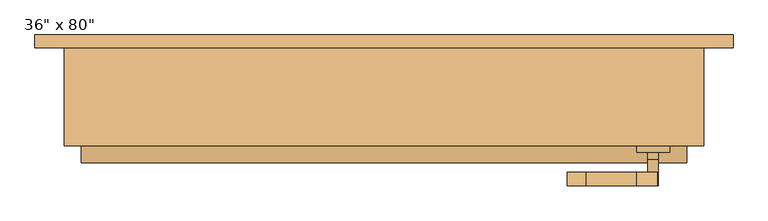
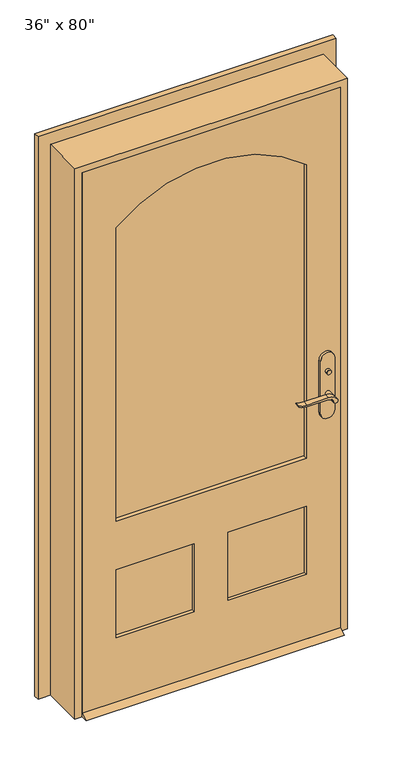
"""IFC4 building model written with IfcOpenShell, lengths in millimetres: door geometry."""

from ifc_helpers import new_model, si_unit, point, frame, frame_2d, origin, place, context, project, spatial, polyline, circle_curve, trimmed, segment, composite_curve, outline, extrude, faceted_brep, source, transform, mapped, element, save


def door_19287a7a(model_context):
    return source(origin(), model_context, "Body", "SolidModel", [
        extrude(outline(polyline([(-33.9718823, 12.7), (-8.5718823, 0.0), (-94.2968823, 0.0), (-68.8968823, 12.7), (-33.9718823, 12.7)])), frame((-457.2, 0.0, 0.0), z_axis=(1.0, 0.0, 0.0), x_axis=(0.0, 1.0, 0.0)), (0.0, 0.0, 1.0), 914.4),
        extrude(outline(polyline([(411.4, -13.9718823), (411.4, -23.9718823), (401.4, -23.9718823), (401.4, -13.9718823), (411.4, -13.9718823)])), frame((0.0, 0.0, 981.9), z_axis=(0.0, 0.0, 1.0), x_axis=(1.0, 0.0, 0.0)), (0.0, 0.0, 1.0), 30.0),
        extrude(outline(composite_curve([segment(trimmed(circle_curve(frame_2d((996.9, 406.4)), 8.0), [point((996.9, 398.4))], [point((996.9, 414.4))], False, "CARTESIAN"), True, "CONTINUOUS"), segment(trimmed(circle_curve(frame_2d((996.9, 406.4)), 8.0), [point((996.9, 414.4))], [point((996.9, 398.4))], False, "CARTESIAN"), True, "CONTINUOUS")], self_intersect=False)), frame((0.0, -88.8968823, 0.0), z_axis=(0.0, 1.0, 0.0), x_axis=(0.0, 0.0, 1.0)), (0.0, 0.0, 1.0), 10.0),
        extrude(outline(composite_curve([segment(trimmed(circle_curve(frame_2d((897.1555521, 382.7324871)), 37.2832219), [point((919.0523287, 412.9081363))], [point((934.4, 381.0325667))], False, "CARTESIAN"), True, "CONTINUOUS"), segment(polyline([(934.4, 381.0325667), (934.4, 304.7564091)]), True, "CONTINUOUS"), segment(trimmed(circle_curve(frame_2d((1017.6850638, 304.8227909)), 83.2850902), [point((934.4, 304.7564091))], [point((939.4, 276.4))], True, "CARTESIAN"), True, "CONTINUOUS"), segment(polyline([(939.4, 276.4), (936.6135558, 276.4)]), True, "CONTINUOUS"), segment(trimmed(circle_curve(frame_2d((986.6709207, 308.3396612)), 59.3791355), [point((936.6135558, 276.4))], [point((927.4, 304.7564091))], False, "CARTESIAN"), True, "CONTINUOUS"), segment(polyline([(927.4, 304.7564091), (927.4, 381.0138099)]), True, "CONTINUOUS"), segment(trimmed(circle_curve(frame_2d((909.2738613, 381.0138099)), 18.1261387), [point((927.4, 381.0138099))], [point((914.4, 398.4))], True, "CARTESIAN"), True, "CONTINUOUS"), segment(trimmed(circle_curve(frame_2d((914.4, 406.4)), 8.0), [point((914.4, 398.4))], [point((919.0523287, 412.9081363))], False, "CARTESIAN"), True, "CONTINUOUS")], self_intersect=False)), frame((0.0, 6.0281177, 0.0), z_axis=(0.0, 1.0, 0.0), x_axis=(0.0, 0.0, 1.0)), (0.0, 0.0, 1.0), 20.0),
        extrude(outline(composite_curve([segment(trimmed(circle_curve(frame_2d((914.4, 406.4)), 8.0), [point((914.3999903, 398.4))], [point((919.0523287, 412.9081363))], False, "CARTESIAN"), True, "CONTINUOUS"), segment(trimmed(circle_curve(frame_2d((897.1555521, 382.7324871)), 37.2832219), [point((919.0523287, 412.9081363))], [point((934.4, 381.0325667))], False, "CARTESIAN"), True, "CONTINUOUS"), segment(polyline([(934.4, 381.0325667), (934.4, 304.7564091)]), True, "CONTINUOUS"), segment(trimmed(circle_curve(frame_2d((1017.6850638, 304.8227909)), 83.2850902), [point((934.4, 304.7564091))], [point((939.4, 276.4))], True, "CARTESIAN"), True, "CONTINUOUS"), segment(polyline([(939.4, 276.4), (936.6135558, 276.4)]), True, "CONTINUOUS"), segment(trimmed(circle_curve(frame_2d((986.6709207, 308.3396612)), 59.3791355), [point((936.6135558, 276.4))], [point((927.4, 304.7564091))], False, "CARTESIAN"), True, "CONTINUOUS"), segment(polyline([(927.4, 304.7564091), (927.4, 381.0138122)]), True, "CONTINUOUS"), segment(trimmed(circle_curve(frame_2d((909.2738682, 381.0138122)), 18.1261318), [point((927.4, 381.0138122))], [point((914.3999903, 398.4))], True, "CARTESIAN"), True, "CONTINUOUS")], self_intersect=False)), frame((0.0, -128.8968823, 0.0), z_axis=(0.0, 1.0, 0.0), x_axis=(0.0, 0.0, 1.0)), (0.0, 0.0, 1.0), 20.0),
        extrude(outline(composite_curve([segment(trimmed(circle_curve(frame_2d((914.4, 406.4)), 8.0), [point((914.4, 398.4))], [point((914.4, 414.4))], False, "CARTESIAN"), True, "CONTINUOUS"), segment(trimmed(circle_curve(frame_2d((914.4, 406.4)), 8.0), [point((914.4, 414.4))], [point((914.4, 398.4))], False, "CARTESIAN"), True, "CONTINUOUS")], self_intersect=False)), frame((0.0, -23.9718823, 0.0), z_axis=(0.0, 1.0, 0.0), x_axis=(0.0, 0.0, 1.0)), (0.0, 0.0, 1.0), 30.0),
        extrude(outline(composite_curve([segment(trimmed(circle_curve(frame_2d((914.4, 406.4)), 8.0), [point((914.4, 398.4))], [point((914.4, 414.4))], False, "CARTESIAN"), True, "CONTINUOUS"), segment(trimmed(circle_curve(frame_2d((914.4, 406.4)), 8.0), [point((914.4, 414.4))], [point((914.4, 398.4))], False, "CARTESIAN"), True, "CONTINUOUS")], self_intersect=False)), frame((0.0, -108.8968823, 0.0), z_axis=(0.0, 1.0, 0.0), x_axis=(0.0, 0.0, 1.0)), (0.0, 0.0, 1.0), 30.0),
        extrude(outline(composite_curve([segment(polyline([(844.4, 431.4), (1039.4, 431.4)]), True, "CONTINUOUS"), segment(trimmed(circle_curve(frame_2d((1039.4, 406.4)), 25.0), [point((1039.4, 431.4))], [point((1039.4, 381.4))], False, "CARTESIAN"), True, "CONTINUOUS"), segment(polyline([(1039.4, 381.4), (844.4, 381.4)]), True, "CONTINUOUS"), segment(trimmed(circle_curve(frame_2d((844.4, 406.4)), 25.0), [point((844.4, 381.4))], [point((844.4, 431.4))], False, "CARTESIAN"), True, "CONTINUOUS")], self_intersect=False)), frame((0.0, -33.9718823, 0.0), z_axis=(0.0, 1.0, 0.0), x_axis=(0.0, 0.0, 1.0)), (0.0, 0.0, 1.0), 10.0),
        extrude(outline(composite_curve([segment(polyline([(844.4, 431.4), (1039.4, 431.4)]), True, "CONTINUOUS"), segment(trimmed(circle_curve(frame_2d((1039.4, 406.4)), 25.0), [point((1039.4, 431.4))], [point((1039.4, 381.4))], False, "CARTESIAN"), True, "CONTINUOUS"), segment(polyline([(1039.4, 381.4), (844.4, 381.4)]), True, "CONTINUOUS"), segment(trimmed(circle_curve(frame_2d((844.4, 406.4)), 25.0), [point((844.4, 381.4))], [point((844.4, 431.4))], False, "CARTESIAN"), True, "CONTINUOUS")], self_intersect=False)), frame((0.0, -78.8968823, 0.0), z_axis=(0.0, 1.0, 0.0), x_axis=(0.0, 0.0, 1.0)), (0.0, 0.0, 1.0), 10.0),
        extrude(outline(polyline([(2032.0, -457.2), (12.7, -457.2), (12.7, 457.2), (2032.0, 457.2), (2032.0, -457.2)]), holes=[composite_curve([segment(polyline([(688.975, -336.55), (1784.35, -336.55)]), True, "CONTINUOUS"), segment(trimmed(circle_curve(frame_2d((1401.92125, 0.0)), 509.42875), [point((1784.35, -336.55))], [point((1784.35, 336.55))], True, "CARTESIAN"), True, "CONTINUOUS"), segment(polyline([(1784.35, 336.55), (688.975, 336.55), (688.975, -336.55)]), True, "CONTINUOUS")], self_intersect=False), polyline([(508.0, -60.325), (254.0, -60.325), (254.0, -336.55), (508.0, -336.55), (508.0, -60.325)]), polyline([(508.0, 336.55), (254.0, 336.55), (254.0, 60.325), (508.0, 60.325), (508.0, 336.55)])]), frame((0.0, -68.8968823, 0.0), z_axis=(0.0, 1.0, 0.0), x_axis=(0.0, 0.0, 1.0)), (0.0, 0.0, 1.0), 34.925),
        faceted_brep([(482.6, -68.8968823, 0.0), (457.2, -68.8968823, 0.0), (457.2, -33.9718823, 0.0), (444.5, -33.9718823, 0.0), (444.5, 0.9531177, 0.0), (457.2, 0.9531177, 0.0), (457.2, 79.375, 0.0), (482.6, 79.375, 0.0), (482.6, 79.375, 2057.4), (482.6, -68.8968823, 2057.4), (457.2, 79.375, 2032.0), (-457.2, 79.375, 2032.0), (-457.2, 79.375, 0.0), (-482.6, 79.375, 0.0), (-482.6, 79.375, 2057.4), (457.2, 0.9531177, 2032.0), (444.5, 0.9531177, 2019.3), (-444.5, 0.9531177, 2019.3), (-444.5, 0.9531177, 0.0), (-457.2, 0.9531177, 0.0), (-457.2, 0.9531177, 2032.0), (444.5, -33.9718823, 2019.3), (457.2, -33.9718823, 2032.0), (-457.2, -33.9718823, 2032.0), (-457.2, -33.9718823, 0.0), (-444.5, -33.9718823, 0.0), (-444.5, -33.9718823, 2019.3), (457.2, -68.8968823, 2032.0), (-482.6, -68.8968823, 2057.4), (-482.6, -68.8968823, 0.0), (-457.2, -68.8968823, 0.0), (-457.2, -68.8968823, 2032.0)], [[[0, 1, 2, 3, 4, 5, 6, 7]], [[7, 8, 9, 0]], [[6, 10, 11, 12, 13, 14, 8, 7]], [[5, 15, 10, 6]], [[4, 16, 17, 18, 19, 20, 15, 5]], [[3, 21, 16, 4]], [[2, 22, 23, 24, 25, 26, 21, 3]], [[1, 27, 22, 2]], [[0, 9, 28, 29, 30, 31, 27, 1]], [[8, 14, 28, 9]], [[15, 20, 11, 10]], [[21, 26, 17, 16]], [[27, 31, 23, 22]], [[29, 13, 12, 19, 18, 25, 24, 30]], [[14, 13, 29, 28]], [[20, 19, 12, 11]], [[26, 25, 18, 17]], [[31, 30, 24, 23]]]),
        extrude(outline(polyline([(-60.325, -45.613549), (-60.325, -57.2552157), (-336.55, -57.2552157), (-336.55, -45.613549), (-60.325, -45.613549)])), frame((0.0, 0.0, 254.0), z_axis=(0.0, 0.0, 1.0), x_axis=(1.0, 0.0, 0.0)), (0.0, 0.0, 1.0), 254.0),
        extrude(outline(polyline([(336.55, -45.613549), (336.55, -57.2552157), (60.325, -57.2552157), (60.325, -45.613549), (336.55, -45.613549)])), frame((0.0, 0.0, 254.0), z_axis=(0.0, 0.0, 1.0), x_axis=(1.0, 0.0, 0.0)), (0.0, 0.0, 1.0), 254.0),
        extrude(outline(composite_curve([segment(polyline([(688.975, -336.55), (688.975, 336.55), (1784.35, 336.55)]), True, "CONTINUOUS"), segment(trimmed(circle_curve(frame_2d((1401.92125, 0.0)), 509.42875), [point((1784.35, 336.55))], [point((1784.35, -336.55))], False, "CARTESIAN"), True, "CONTINUOUS"), segment(polyline([(1784.35, -336.55), (688.975, -336.55)]), True, "CONTINUOUS")], self_intersect=False)), frame((0.0, -54.9268823, 0.0), z_axis=(0.0, 1.0, 0.0), x_axis=(0.0, 0.0, 1.0)), (0.0, 0.0, 1.0), 6.985),
        extrude(outline(polyline([(0.0, -463.55), (2038.35, -463.55), (2038.35, 463.55), (0.0, 463.55), (0.0, 527.05), (2101.85, 527.05), (2101.85, -527.05), (0.0, -527.05), (0.0, -463.55)])), frame((0.0, 79.375, 0.0), z_axis=(0.0, 1.0, 0.0), x_axis=(0.0, 0.0, 1.0)), (0.0, 0.0, 1.0), 19.05),
    ])


if __name__ == "__main__":
    model = new_model("IFC4")
    model_context = context("Model", 3, world=origin())
    ifc_project = project(units=[si_unit("LENGTHUNIT", "METRE", prefix="MILLI")], contexts=[model_context])
    site = spatial("IfcSite", under=ifc_project)
    building = spatial("IfcBuilding", under=site)
    placement = place(None, origin())
    door_shape = door_19287a7a(model_context)
    element("IfcDoor", 1, ObjectType="36\" x 80\"", at=placement, inside=building, context=model_context, shape_type="MappedRepresentation", body=[
        mapped(door_shape, transform((0.0, 0.0, 0.0), x_axis=(1.0, 0.0, 0.0), y_axis=(0.0, 1.0, 0.0), z_axis=(0.0, 0.0, 1.0))),
    ])
    save(model, "model.ifc")

# Revit data of these elements
# Type "36\" x 80\""
#   Type Mark = "8"
#   Assembly Code = "B2030100"
#   Analytic Construction = "French door, wood frame with single glass"
#   Threshold Offset [instance default] = 0' - 0 1/2"
#   Thickness = 0' - 1 3/8"
#   Thermal Resistance (R) = 1.0696 (h·ft²·°F)/BTU
#   Swing Angle [instance default] = 90.00°
#   Stiles = 0' - 4 3/4"
#   Rough Width = 3' - 2"
#   Rough Height = 6' - 9"
#   Radius = 1' - 8.05625"
#   Lock Rail = 0' - 7 1/8"
#   Height = 6' - 8"
#   Width = 3' - 0"
#   Heat Transfer Coefficient (U) = 0.9350 BTU/(h·ft²·°F)
#   Door Offset [instance default] = 0' - 0"
#   Bottom Rail = 0' - 9 1/2"
#   Threshold [instance default] = yes
#   Function = 1
#   Exterior Trim [instance default] = yes
#   Trim Material = Cherry
#   Threshold Material = Cherry
#   Panel Material = Cherry
#   Glazing = Glass
#   Frame Material = Cherry
#   Door Handle Material = Aluminum
#   Visual Light Transmittance = 0
#   Solar Heat Gain Coefficient = 0
#   Wall Closure = (empty or 0)
#   Construction Type = (empty or 0)
# Element 1 (IfcDoor, "36\" x 80\"")
#   Door Offset = 0' - 0.16252"
#   Exterior Trim = no
#   Materials on its faces: "Cherry", "Aluminum", "Glass"
# Materials
#   "Cherry": class "Wood", colour RGB 226 177 128, transparency 0, Description = "Prunus Serotina", Cost = 0
#   "Glass": class "Glass", colour RGB 0 128 192, transparency 0.75, Description = "Soda Lime Glass", Cost = 0
#   "Aluminum": class "Metal", colour RGB 247 247 247, transparency 0, Description = "Aluminum 6061", Cost = 0
